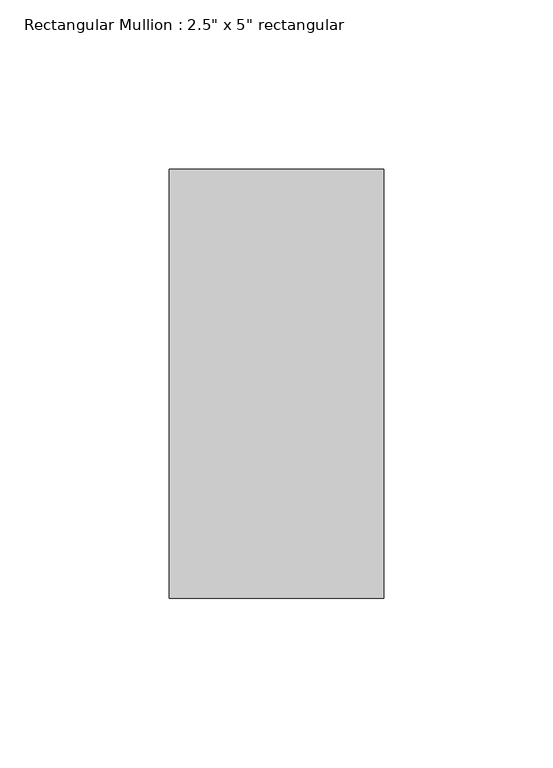
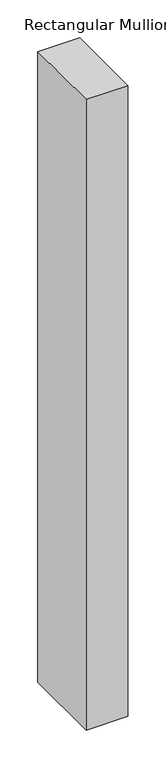
"""IFC4 building model written with IfcOpenShell, lengths in millimetres: member geometry."""

from ifc_helpers import new_model, si_unit, frame, origin, place, context, project, spatial, polyline, outline, extrude, source, transform, mapped, element, save


def member_8e09d03a(model_context):
    return source(origin(), model_context, "Body", "SweptSolid", [
        extrude(outline(polyline([(0.0, 63.5), (0.0, -63.5), (-63.5, -63.5), (-63.5, 63.5), (0.0, 63.5)])), frame((0.0, 0.0, -1016.0), z_axis=(0.0, 0.0, 1.0), x_axis=(1.0, 0.0, 0.0)), (0.0, 0.0, 1.0), 1016.0),
    ])


if __name__ == "__main__":
    model = new_model("IFC4")
    model_context = context("Model", 3, world=origin())
    ifc_project = project(units=[si_unit("LENGTHUNIT", "METRE", prefix="MILLI")], contexts=[model_context])
    site = spatial("IfcSite", under=ifc_project)
    building = spatial("IfcBuilding", under=site)
    placement = place(None, origin())
    member_shape = member_8e09d03a(model_context)
    element("IfcMember", 1, ObjectType="Rectangular Mullion : 2.5\" x 5\" rectangular", at=placement, inside=building, context=model_context, shape_type="MappedRepresentation", body=[
        mapped(member_shape, transform((0.0, 0.0, 0.0), x_axis=(1.0, 0.0, 0.0), y_axis=(0.0, 1.0, 0.0), z_axis=(0.0, 0.0, 1.0))),
    ])
    save(model, "model.ifc")

# Revit data of these elements
# Type "Rectangular Mullion : 2.5\" x 5\" rectangular"
#   built-in parameter 1007304 = 0.416667 (stored number, unit not read)
#   built-in parameter 1007301 = 0.104167 (stored number, unit not read)
#   built-in parameter 1007300 = 0.104167 (stored number, unit not read)
